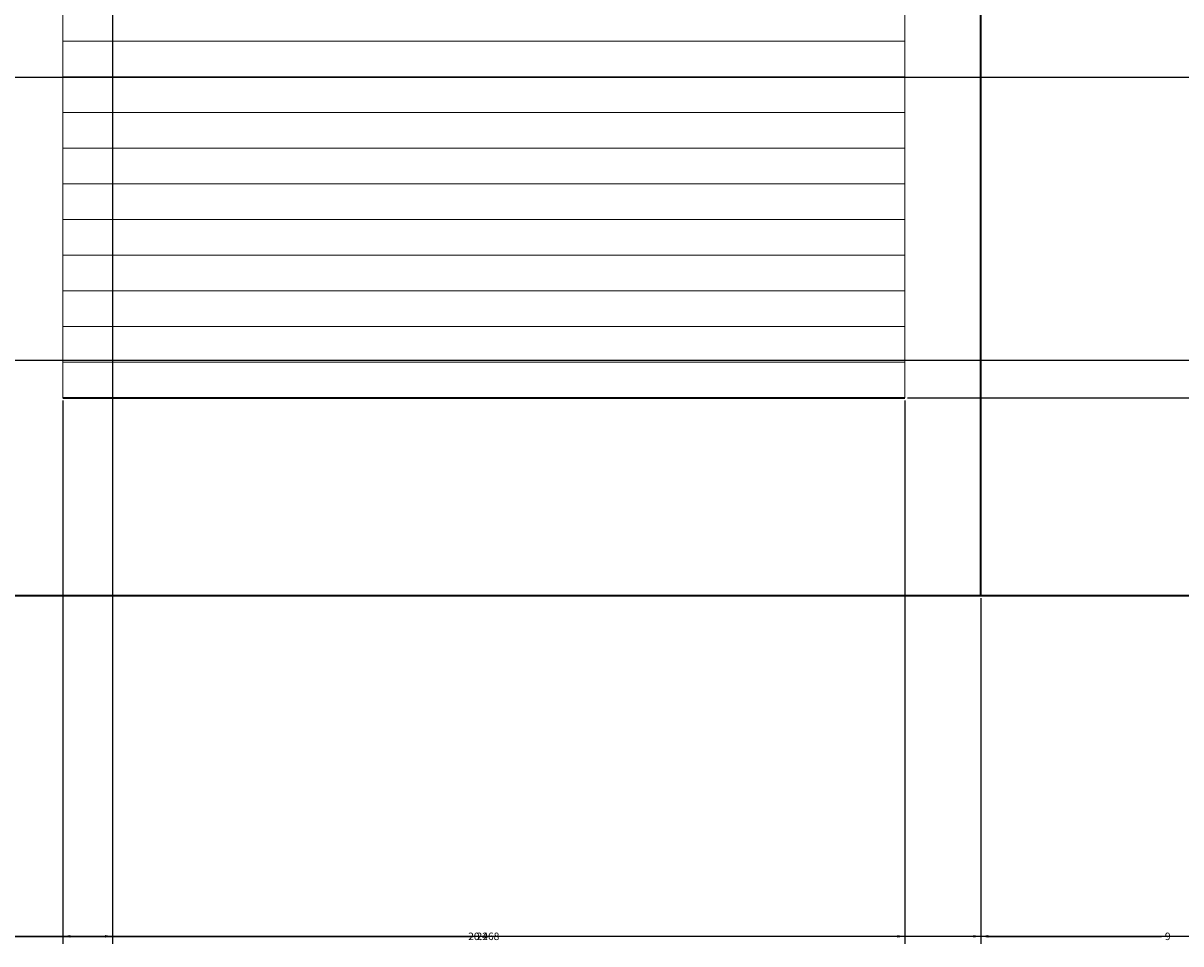
# Model space of a CAD drawing. Units: inches. Extents: x 27 to 200, y -50 to 102.
# Tile 12 of 26: x 144 to 172, y -25 to -3. Entities that reach past the tile are written whole.
import ezdxf

# ---------------------------------------------------------------- set-up
doc = ezdxf.new("R2010")
doc.units = ezdxf.units.IN
doc.header["$MEASUREMENT"] = 0
for name, color, linetype, lineweight in [('A-ANNO-DIMS', 2, 'Continuous', 18), ('A-ELEV', 7, 'Continuous', 35), ('A-EQPM', 9, 'Continuous', 18), ('A-FURN', 8, 'Continuous', 18)]:
    doc.layers.add(name, color=color, linetype=linetype, lineweight=lineweight)
doc.styles.get("Standard").update_dxf_attribs({"font": 'arial.ttf'})
doc.dimstyles.get("Standard").update_dxf_attribs({"dimtxt": 0.18, "dimasz": 0.18, "dimexe": 0.18, "dimexo": 0.0625, "dimgap": 0.09, "dimtad": 0, "dimtih": 1, "dimtoh": 1, "dimdec": 4, "dimzin": 0, "dimdsep": 46, "dimtxsty": 'Standard', "dimcen": 0.09, "dimadec": 0, "dimazin": 0, "dimtfac": 1, "dimtdec": 4, "dimtofl": 0, "dimtmove": 0, "dimatfit": 3, "dimfxl": 1, "dimtolj": 1, "dimtzin": 0, "dimarcsym": 0})

# ---------------------------------------------------------------- blocks, each defined once
blk = doc.blocks.new('*D23')
at = {"layer": 'A-ANNO-DIMS', "color": 0, "lineweight": -2, "transparency": 16777216}
for p, q in [((35.417, -16.832), (35.417, -25.149)), ((191.417, -16.832), (191.417, -25.149)), ((35.597, -24.969), (113.137, -24.969)), ((191.237, -24.969), (113.697, -24.969))]:
    blk.add_line(p, q, dxfattribs=at)
at = {"layer": 'A-ANNO-DIMS', "color": 0, "transparency": 16777216}
for points in [[(35.597, -24.939), (35.597, -24.999), (35.417, -24.969)], [(191.237, -24.939), (191.237, -24.999), (191.417, -24.969)]]:
    blk.add_solid(points, dxfattribs=at)
at = {"layer": 'Defpoints', "color": 0, "transparency": 16777216}
for p in [(35.417, -16.769), (191.417, -16.769), (191.417, -24.969)]:
    blk.add_point(p, dxfattribs=at)
at = {"layer": 'A-ANNO-DIMS', "color": 0, "transparency": 16777216, "insert": (113.417, -24.969), "char_height": 0.18, "attachment_point": 5}
blk.add_mtext('\\A1;156', dxfattribs=at)
blk = doc.blocks.new('*D38')
at = {"layer": 'A-ANNO-DIMS', "color": 0, "lineweight": -2, "transparency": 16777216}
for p, q in [((143.312, -16.832), (143.312, -25.149)), ((167.312, -16.832), (167.312, -25.149)), ((143.492, -24.969), (155.092, -24.969)), ((167.132, -24.969), (155.532, -24.969))]:
    blk.add_line(p, q, dxfattribs=at)
at = {"layer": 'A-ANNO-DIMS', "color": 0, "transparency": 16777216}
for points in [[(143.492, -24.939), (143.492, -24.999), (143.312, -24.969)], [(167.132, -24.939), (167.132, -24.999), (167.312, -24.969)]]:
    blk.add_solid(points, dxfattribs=at)
at = {"layer": 'Defpoints', "color": 0, "transparency": 16777216}
for p in [(143.312, -16.769), (167.312, -16.769), (167.312, -24.969)]:
    blk.add_point(p, dxfattribs=at)
at = {"layer": 'A-ANNO-DIMS', "color": 0, "transparency": 16777216, "insert": (155.312, -24.969), "char_height": 0.18, "attachment_point": 5}
blk.add_mtext('\\A1;24', dxfattribs=at)
blk = doc.blocks.new('*D39')
at = {"layer": 'A-ANNO-DIMS', "color": 0, "lineweight": -2, "transparency": 16777216}
for p, q in [((167.312, -16.832), (167.312, -25.149)), ((176.312, -16.832), (176.312, -25.149)), ((167.492, -24.969), (171.663, -24.969)), ((176.132, -24.969), (171.961, -24.969))]:
    blk.add_line(p, q, dxfattribs=at)
at = {"layer": 'A-ANNO-DIMS', "color": 0, "transparency": 16777216}
for points in [[(167.492, -24.939), (167.492, -24.999), (167.312, -24.969)], [(176.132, -24.939), (176.132, -24.999), (176.312, -24.969)]]:
    blk.add_solid(points, dxfattribs=at)
at = {"layer": 'Defpoints', "color": 0, "transparency": 16777216}
for p in [(167.312, -16.769), (176.312, -16.769), (176.312, -24.969)]:
    blk.add_point(p, dxfattribs=at)
at = {"layer": 'A-ANNO-DIMS', "color": 0, "transparency": 16777216, "insert": (171.812, -24.969), "char_height": 0.18, "attachment_point": 5}
blk.add_mtext('\\A1;9', dxfattribs=at)
blk = doc.blocks.new('*D48')
at = {"layer": 'A-ANNO-DIMS', "color": 0, "lineweight": -2, "transparency": 16777216}
for p, q in [((84.479, 44.926), (199.797, 44.926)), ((199.617, 44.746), (199.617, 14.26)), ((199.617, -16.589), (199.617, 13.897)), ((84.479, -16.769), (199.797, -16.769))]:
    blk.add_line(p, q, dxfattribs=at)
at = {"layer": 'A-ANNO-DIMS', "color": 0, "transparency": 16777216}
for points in [[(199.587, 44.746), (199.647, 44.746), (199.617, 44.926)], [(199.587, -16.589), (199.647, -16.589), (199.617, -16.769)]]:
    blk.add_solid(points, dxfattribs=at)
at = {"layer": 'Defpoints', "color": 0, "transparency": 16777216}
for p in [(84.417, 44.926), (199.617, 44.926), (84.417, -16.769)]:
    blk.add_point(p, dxfattribs=at)
at = {"layer": 'A-ANNO-DIMS', "color": 0, "transparency": 16777216, "insert": (199.617, 14.079), "char_height": 0.18, "attachment_point": 5}
blk.add_mtext('\\A1;61.7', dxfattribs=at)
blk = doc.blocks.new('*D51')
at = {"layer": 'A-ANNO-DIMS', "color": 0, "lineweight": -2, "transparency": 16777216}
for p, q in [((120.417, 45.561), (120.417, -25.149)), ((146.417, 45.561), (146.417, -25.149)), ((120.597, -24.969), (133.197, -24.969)), ((146.237, -24.969), (133.637, -24.969))]:
    blk.add_line(p, q, dxfattribs=at)
at = {"layer": 'A-ANNO-DIMS', "color": 0, "transparency": 16777216}
for points in [[(120.597, -24.939), (120.597, -24.999), (120.417, -24.969)], [(146.237, -24.939), (146.237, -24.999), (146.417, -24.969)]]:
    blk.add_solid(points, dxfattribs=at)
at = {"layer": 'Defpoints', "color": 0, "transparency": 16777216}
for p in [(120.417, 45.623), (146.417, 45.623), (146.417, -24.969)]:
    blk.add_point(p, dxfattribs=at)
at = {"layer": 'A-ANNO-DIMS', "color": 0, "transparency": 16777216, "insert": (133.417, -24.969), "char_height": 0.18, "attachment_point": 5}
blk.add_mtext('\\A1;26', dxfattribs=at)
blk = doc.blocks.new('*D62')
at = {"layer": 'A-ANNO-DIMS', "color": 0, "lineweight": -2, "transparency": 16777216}
for p, q in [((140.41, -4.3), (199.797, -4.3)), ((199.617, -4.48), (199.617, -7.522)), ((199.617, -10.928), (199.617, -7.886)), ((140.41, -11.108), (199.797, -11.108))]:
    blk.add_line(p, q, dxfattribs=at)
at = {"layer": 'A-ANNO-DIMS', "color": 0, "transparency": 16777216}
for points in [[(199.587, -4.48), (199.647, -4.48), (199.617, -4.3)], [(199.587, -10.928), (199.647, -10.928), (199.617, -11.108)]]:
    blk.add_solid(points, dxfattribs=at)
at = {"layer": 'Defpoints', "color": 0, "transparency": 16777216}
for p in [(140.347, -4.3), (199.617, -4.3), (140.347, -11.108)]:
    blk.add_point(p, dxfattribs=at)
at = {"layer": 'A-ANNO-DIMS', "color": 0, "transparency": 16777216, "insert": (199.617, -7.704), "char_height": 0.18, "attachment_point": 5}
blk.add_mtext('\\A1;6.809', dxfattribs=at)
blk = doc.blocks.new('*D66')
at = {"layer": 'A-ANNO-DIMS', "color": 0, "lineweight": -2, "transparency": 16777216}
for p, q in [((145.216, -12.082), (145.216, -25.149)), ((165.484, -12.082), (165.484, -25.149)), ((145.396, -24.969), (154.885, -24.969)), ((165.304, -24.969), (155.815, -24.969))]:
    blk.add_line(p, q, dxfattribs=at)
at = {"layer": 'A-ANNO-DIMS', "color": 0, "transparency": 16777216}
for points in [[(145.396, -24.939), (145.396, -24.999), (145.216, -24.969)], [(165.304, -24.939), (165.304, -24.999), (165.484, -24.969)]]:
    blk.add_solid(points, dxfattribs=at)
at = {"layer": 'Defpoints', "color": 0, "transparency": 16777216}
for p in [(145.216, -12.019), (165.484, -12.019), (165.484, -24.969)]:
    blk.add_point(p, dxfattribs=at)
at = {"layer": 'A-ANNO-DIMS', "color": 0, "transparency": 16777216, "insert": (155.35, -24.969), "char_height": 0.18, "attachment_point": 5}
blk.add_mtext('\\A1;20.268', dxfattribs=at)
blk = doc.blocks.new('*D67')
at = {"layer": 'A-ANNO-DIMS', "color": 0, "lineweight": -2, "transparency": 16777216}
for p, q in [((165.546, 5.617), (199.797, 5.617)), ((199.617, 5.437), (199.617, -3.019)), ((199.617, -11.839), (199.617, -3.383)), ((165.546, -12.019), (199.797, -12.019))]:
    blk.add_line(p, q, dxfattribs=at)
at = {"layer": 'A-ANNO-DIMS', "color": 0, "transparency": 16777216}
for points in [[(199.587, 5.437), (199.647, 5.437), (199.617, 5.617)], [(199.587, -11.839), (199.647, -11.839), (199.617, -12.019)]]:
    blk.add_solid(points, dxfattribs=at)
at = {"layer": 'Defpoints', "color": 0, "transparency": 16777216}
for p in [(165.484, 5.617), (199.617, 5.617), (165.484, -12.019)]:
    blk.add_point(p, dxfattribs=at)
at = {"layer": 'A-ANNO-DIMS', "color": 0, "transparency": 16777216, "insert": (199.617, -3.201), "char_height": 0.18, "attachment_point": 5}
blk.add_mtext('\\A1;17.636', dxfattribs=at)

msp = doc.modelspace()

# ---------------------------------------------------------------- linework, layer by layer
at = {"layer": 'A-ELEV'}
for p, q in [((167.3118, -16.7693), (167.3118, 16.056)), ((145.216, -12.0191), (165.4839, -12.0191)), ((35.4169, -16.7693), (191.4169, -16.7693))]:
    msp.add_line(p, q, dxfattribs=at)
at = {"layer": 'A-EQPM'}
for p, q in [((145.216, -3.4322), (165.4839, -3.4322)), ((145.216, -4.2909), (165.4839, -4.2909)), ((145.216, -5.1496), (165.4839, -5.1496)), ((145.216, -6.0083), (165.4839, -6.0083)), ((145.216, -6.867), (165.4839, -6.867)), ((145.216, -7.7256), (165.4839, -7.7256)), ((145.216, -8.5843), (165.4839, -8.5843)), ((145.216, -9.443), (165.4839, -9.443)), ((145.216, -10.3017), (165.4839, -10.3017)), ((145.216, -11.1604), (165.4839, -11.1604))]:
    msp.add_line(p, q, dxfattribs=at)
at = {"layer": 'A-FURN'}
msp.add_lwpolyline([(145.216, 5.6167), (165.4839, 5.6167), (165.4839, -12.0191), (145.216, -12.0191)], close=True, dxfattribs=at)

# ---------------------------------------------------------------- dimensions: what is measured, and where the dimension line sits
at = {"layer": 'A-ANNO-DIMS'}
for base, p1, p2, override, picture, middle in [((146.4169, -24.9693), (120.4169, 45.6231), (146.4169, 45.6231), {"dimdec": 0, "dimlfac": 1, "dimrnd": 0, "dimzin": 0, "dimdsep": 46, "dimlunit": 2}, '*D51', (133.4169, -24.9693)), ((165.4839, -24.9693), (145.216, -12.0191), (165.4839, -12.0191), {"dimdec": 3, "dimlfac": 1, "dimrnd": 0, "dimzin": 0, "dimdsep": 46, "dimlunit": 2}, '*D66', (155.3499, -24.9693)), ((191.4169, -24.9693), (35.4169, -16.7693), (191.4169, -16.7693), {"dimdec": 0, "dimlfac": 1, "dimrnd": 0, "dimzin": 0, "dimdsep": 46, "dimlunit": 2}, '*D23', (113.4169, -24.9693)), ((167.3118, -24.9693), (143.3118, -16.7693), (167.3118, -16.7693), {"dimdec": 0, "dimlfac": 1, "dimrnd": 0, "dimzin": 0, "dimdsep": 46, "dimlunit": 2}, '*D38', (155.3118, -24.9693)), ((176.3118, -24.9693), (167.3118, -16.7693), (176.3118, -16.7693), {"dimdec": 0, "dimlfac": 1, "dimrnd": 0, "dimzin": 0, "dimdsep": 46, "dimlunit": 2}, '*D39', (171.8118, -24.9693))]:
    dim = msp.add_linear_dim(base=base, p1=p1, p2=p2, dimstyle='Standard', override=override, dxfattribs=at)
    dim.commit()
    dim.dimension.update_dxf_attribs({"geometry": picture, "text_midpoint": middle})
for base, p1, p2, override, picture, middle in [((199.6169, 44.9264), (84.4169, -16.7693), (84.4169, 44.9264), {"dimdec": 1, "dimlfac": 1, "dimrnd": 0, "dimzin": 0, "dimdsep": 46, "dimlunit": 2}, '*D48', (199.6169, 14.0786)), ((199.6169, 5.6167), (165.4839, -12.0191), (165.4839, 5.6167), {"dimdec": 3, "dimlfac": 1, "dimrnd": 0, "dimzin": 0, "dimdsep": 46, "dimlunit": 2}, '*D67', (199.6169, -3.2012)), ((199.6169, -4.2997), (140.3471, -11.1085), (140.3471, -4.2997), {"dimdec": 3, "dimlfac": 1, "dimrnd": 0, "dimzin": 0, "dimdsep": 46, "dimlunit": 2}, '*D62', (199.6169, -7.7041))]:
    dim = msp.add_linear_dim(base=base, p1=p1, p2=p2, angle=90, dimstyle='Standard', override=override, dxfattribs=at)
    dim.commit()
    dim.dimension.update_dxf_attribs({"geometry": picture, "text_midpoint": middle})

doc.saveas('drawing.dxf')
